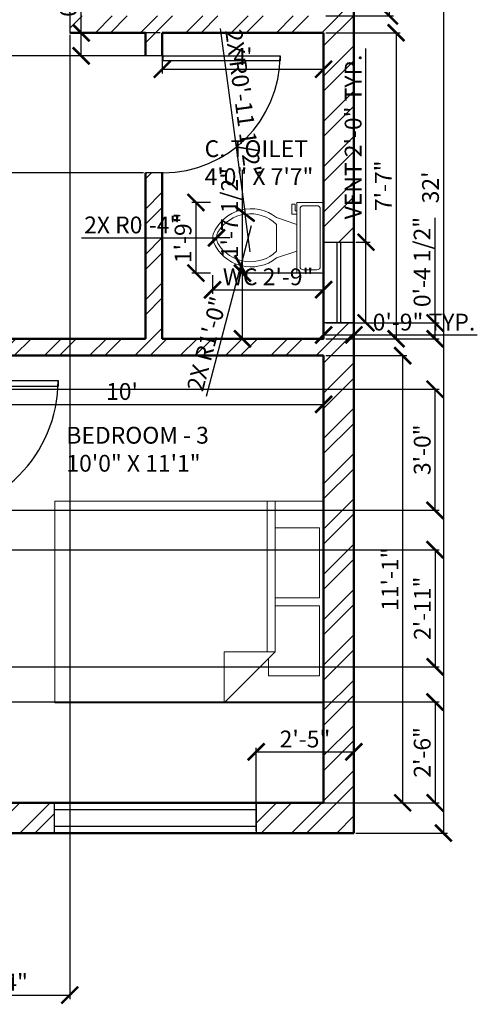
# Model space of a CAD drawing. Units: inches. Extents: x 683 to 1274, y 1901 to 2385.
# Tile 3 of 5: x 930 to 1066, y 1903 to 2196. Entities that reach past the tile are written whole.
import ezdxf

# ---------------------------------------------------------------- set-up
doc = ezdxf.new("R2010")
doc.units = ezdxf.units.IN
for name, color, linetype, lineweight in [('A-AREA-IDEN', 3, 'Continuous', 25), ('A-FLOR-FIXT', 2, 'Continuous', 18), ('A-FURN', 2, 'Continuous', 18), ('A-WALL-PATT', 8, 'Continuous', 13), ('DIM', 3, 'Continuous', 18), ('DOORS', 4, 'Continuous', 25), ('VENTILATOR', 11, 'Continuous', 25), ('walls', 6, 'Continuous', 50), ('WINDOWS', 30, 'Continuous', 25)]:
    doc.layers.add(name, color=color, linetype=linetype, lineweight=lineweight)
doc.styles.get("Standard").update_dxf_attribs({"font": 'arial.ttf'})
doc.dimstyles.new('ISO-25', dxfattribs={"dimtxt": 5, "dimasz": 5, "dimexe": 1.25, "dimexo": 0.625, "dimtad": 1, "dimdec": 1, "dimlunit": 4, "dimtxsty": 'Standard', "dimblk": 'ARCHTICK', "dimcen": 2.5, "dimadec": 0, "dimazin": 0, "dimtfac": 1, "dimtdec": 1, "dimtmove": 0, "dimatfit": 3, "dimfxl": 1, "dimarcsym": 0})

# ---------------------------------------------------------------- blocks, each defined once
blk = doc.blocks.new('Toilet - top')
for p, q in [((9.5, -6), (9.5, -2)), ((-10, -8.5), (-8, -8.5)), ((-10, -9.5), (-10, -8.5)), ((-8, -8.5), (-8, -8)), ((-7, -8), (-7, -9.5)), ((-4, -8), (-6, -14)), ((4, -8), (6, -14)), ((-7, -9.5), (-10, -9.5)), ((4, -14), (-4, -14))]:
    blk.add_line(p, q)
blk.add_lwpolyline([(10.5, -8), (10.5, 0), (-10.5, 0), (-10.5, -8)], close=True)
for points in [[(-9.5, -2), (-9.5, -6)], [(8.5, -1), (-8.5, -1)], [(-8.5, -7), (8.5, -7)]]:
    blk.add_lwpolyline(points)
for centre, radius, start, end in [((-8.62, -1.88), 0.884, 81.8699, 188.1301), ((8.62, -1.88), 0.884, 351.8699, 98.1301), ((-8.62, -6.12), 0.884, 171.8699, 278.1301), ((8.62, -6.12), 0.884, 261.8699, 8.1301), ((3.52, -21.58), 12.17, 141.4691, 247.9714), ((4.2, -21.82), 11.33, 136.3677, 238.9468), ((-3.52, -21.58), 12.17, 292.0284, 38.5307), ((-4.2, -21.82), 11.33, 301.053, 43.6321), ((0, -27.88), 4, 245.7318, 294.2682), ((0, -29), 4, 254.8605, 285.1395)]:
    blk.add_arc(centre, radius, start, end)
blk = doc.blocks.new('Bed - Queen')
for p, q in [((0, -80.00003), (0, 0)), ((0, 0), (59.99999, 0)), ((59.99999, 0), (59.99999, -80.00003)), ((7.99999, -1.2), (28.79998, -1.2)), ((7.99999, -14.4), (7.99999, -1.2)), ((28.79998, -1.2), (28.79998, -14.4)), ((31.19999, -1.2), (51.99999, -1.2)), ((31.19999, -14.4), (31.19999, -1.2)), ((51.99999, -1.2), (51.99999, -16.4)), ((0, -14.4), (44.8, -14.4)), ((59.99999, -29.6), (44.8, -14.4)), ((44.8, -14.4), (44.8, -29.6)), ((44.8, -16.8), (0, -16.8)), ((51.99999, -16.4), (46.79936, -16.4)), ((44.8, -29.6), (59.99999, -29.6)), ((59.99999, -80.00003), (0, -80.00003))]:
    blk.add_line(p, q)
blk = doc.blocks.new('_ArchTick')
at = {"color": 0, "linetype": 'ByBlock', "const_width": 0.15}
blk.add_lwpolyline([(-0.5, -0.5), (0.5, 0.5)], dxfattribs=at)
blk = doc.blocks.new('*D7')
at = {"layer": 'Defpoints', "color": 0, "transparency": 16777216}
for p in [(1029.42, 2337.78), (1029.42, 1953.78), (1056.05, 1953.78)]:
    blk.add_point(p, dxfattribs=at)
at = {"layer": 'DIM', "color": 0, "lineweight": -2, "transparency": 16777216}
for p, q in [((1030.04, 2337.78), (1057.3, 2337.78)), ((1056.05, 2337.78), (1056.05, 1953.78)), ((1030.04, 1953.78), (1057.3, 1953.78))]:
    blk.add_line(p, q, dxfattribs=at)
at = {"layer": 'DIM', "color": 0, "lineweight": -2, "transparency": 16777216, "xscale": 5, "yscale": 5, "zscale": 5}
for p, rotation in [((1056.05, 2337.78), 90), ((1056.05, 1953.78), 270)]:
    blk.add_blockref('_ArchTick', p, dxfattribs=dict(at, rotation=rotation))
at = {"layer": 'DIM', "color": 0, "transparency": 16777216, "insert": (1052.87, 2145.78), "char_height": 5, "attachment_point": 5, "rotation": 90}
blk.add_mtext("32'", dxfattribs=at)
blk = doc.blocks.new('*D8')
at = {"layer": 'Defpoints', "color": 0, "transparency": 16777216}
for p in [(900.42, 2095.78), (1020.42, 2095.78), (1020.42, 2081.28)]:
    blk.add_point(p, dxfattribs=at)
at = {"layer": 'DIM', "color": 0, "lineweight": -2, "transparency": 16777216}
for p, q in [((900.42, 2095.16), (900.42, 2080.03)), ((1020.42, 2095.16), (1020.42, 2080.03)), ((900.42, 2081.28), (1020.42, 2081.28))]:
    blk.add_line(p, q, dxfattribs=at)
at = {"layer": 'DIM', "color": 0, "lineweight": -2, "transparency": 16777216, "xscale": 5, "yscale": 5, "zscale": 5, "rotation": 180}
blk.add_blockref('_ArchTick', (900.42, 2081.28), dxfattribs=at)
at = {"layer": 'DIM', "color": 0, "lineweight": -2, "transparency": 16777216, "xscale": 5, "yscale": 5, "zscale": 5}
blk.add_blockref('_ArchTick', (1020.42, 2081.28), dxfattribs=at)
at = {"layer": 'DIM', "color": 0, "transparency": 16777216, "insert": (960.42, 2084.46), "char_height": 5, "attachment_point": 5}
blk.add_mtext("10'", dxfattribs=at)
blk = doc.blocks.new('*D11')
at = {"layer": 'Defpoints', "color": 0, "transparency": 16777216}
for p in [(972.42, 2191.78), (1020.42, 2191.78), (1020.42, 2180.94)]:
    blk.add_point(p, dxfattribs=at)
at = {"layer": 'DIM', "color": 0, "lineweight": -2, "transparency": 16777216}
for p, q in [((972.42, 2191.16), (972.42, 2179.69)), ((1020.42, 2191.16), (1020.42, 2179.69)), ((972.42, 2180.94), (1020.42, 2180.94))]:
    blk.add_line(p, q, dxfattribs=at)
at = {"layer": 'DIM', "color": 0, "lineweight": -2, "transparency": 16777216, "xscale": 5, "yscale": 5, "zscale": 5, "rotation": 180}
blk.add_blockref('_ArchTick', (972.42, 2180.94), dxfattribs=at)
at = {"layer": 'DIM', "color": 0, "lineweight": -2, "transparency": 16777216, "xscale": 5, "yscale": 5, "zscale": 5}
blk.add_blockref('_ArchTick', (1020.42, 2180.94), dxfattribs=at)
at = {"layer": 'DIM', "color": 0, "transparency": 16777216, "insert": (996.42, 2184.07), "char_height": 5, "attachment_point": 5}
blk.add_mtext("4'", dxfattribs=at)
blk = doc.blocks.new('VENTILATOR')
at = {"layer": 'VENTILATOR'}
for p, q in [((1084.96, 2166.43), (1093.96, 2166.43)), ((1084.96, 2142.43), (1084.96, 2166.43)), ((1088.96, 2142.43), (1088.96, 2166.43)), ((1089.96, 2166.43), (1089.96, 2142.43)), ((1093.96, 2166.43), (1093.96, 2142.43)), ((1093.96, 2142.43), (1084.96, 2142.43))]:
    blk.add_line(p, q, dxfattribs=at)
blk = doc.blocks.new('W1')
at = {"layer": 'WINDOWS'}
for p, q in [((1078.63, 2170.04), (1087.63, 2170.04)), ((1078.63, 2110.04), (1078.63, 2170.04)), ((1080.63, 2110.04), (1080.63, 2170.04)), ((1085.63, 2170.04), (1085.63, 2110.04)), ((1087.63, 2170.04), (1087.63, 2110.04)), ((1087.63, 2110.04), (1078.63, 2110.04))]:
    blk.add_line(p, q, dxfattribs=at)
blk = doc.blocks.new('*U18')
for p, q in [((0, 0), (0, -6)), ((40, 0), (40, -6))]:
    blk.add_line(p, q)
blk.add_lwpolyline([(0, 0), (0, 40), (1.75, 40), (1.75, 0)], close=True)
blk.add_arc((0, 0), 40, 0, 90)
blk = doc.blocks.new('*D20')
at = {"layer": 'Defpoints', "color": 0, "transparency": 16777216}
for p in [(1020.42, 2328.78), (1040, 2328.78), (1020.42, 2196.78)]:
    blk.add_point(p, dxfattribs=at)
at = {"layer": 'DIM', "color": 0, "lineweight": -2, "transparency": 16777216}
for p, q in [((1021.04, 2328.78), (1041.25, 2328.78)), ((1040, 2196.78), (1040, 2328.78)), ((1021.04, 2196.78), (1041.25, 2196.78))]:
    blk.add_line(p, q, dxfattribs=at)
at = {"layer": 'DIM', "color": 0, "lineweight": -2, "transparency": 16777216, "xscale": 5, "yscale": 5, "zscale": 5}
for p, rotation in [((1040, 2328.78), 90), ((1040, 2196.78), 270)]:
    blk.add_blockref('_ArchTick', p, dxfattribs=dict(at, rotation=rotation))
at = {"layer": 'DIM', "color": 0, "transparency": 16777216, "insert": (1036.87, 2262.78), "char_height": 5, "attachment_point": 5, "rotation": 90}
blk.add_mtext("11'", dxfattribs=at)
blk = doc.blocks.new('*D21')
at = {"layer": 'Defpoints', "color": 0, "transparency": 16777216}
for p in [(1020.42, 2191.78), (1020.42, 2100.78), (1041.97, 2100.78)]:
    blk.add_point(p, dxfattribs=at)
at = {"layer": 'DIM', "color": 0, "lineweight": -2, "transparency": 16777216}
for p, q in [((1021.04, 2191.78), (1043.22, 2191.78)), ((1041.97, 2191.78), (1041.97, 2100.78)), ((1021.04, 2100.78), (1043.22, 2100.78))]:
    blk.add_line(p, q, dxfattribs=at)
at = {"layer": 'DIM', "color": 0, "lineweight": -2, "transparency": 16777216, "xscale": 5, "yscale": 5, "zscale": 5}
for p, rotation in [((1041.97, 2191.78), 90), ((1041.97, 2100.78), 270)]:
    blk.add_blockref('_ArchTick', p, dxfattribs=dict(at, rotation=rotation))
at = {"layer": 'DIM', "color": 0, "transparency": 16777216, "insert": (1038.84, 2146.28), "char_height": 5, "attachment_point": 5, "rotation": 90}
blk.add_mtext('7\'-7"', dxfattribs=at)
blk = doc.blocks.new('*D22')
at = {"layer": 'Defpoints', "color": 0, "transparency": 16777216}
for p in [(1020.42, 2095.78), (1020.42, 1962.78), (1043.93, 1962.78)]:
    blk.add_point(p, dxfattribs=at)
at = {"layer": 'DIM', "color": 0, "lineweight": -2, "transparency": 16777216}
for p, q in [((1021.04, 2095.78), (1045.18, 2095.78)), ((1043.93, 2095.78), (1043.93, 1962.78)), ((1021.04, 1962.78), (1045.18, 1962.78))]:
    blk.add_line(p, q, dxfattribs=at)
at = {"layer": 'DIM', "color": 0, "lineweight": -2, "transparency": 16777216, "xscale": 5, "yscale": 5, "zscale": 5}
for p, rotation in [((1043.93, 2095.78), 90), ((1043.93, 1962.78), 270)]:
    blk.add_blockref('_ArchTick', p, dxfattribs=dict(at, rotation=rotation))
at = {"layer": 'DIM', "color": 0, "transparency": 16777216, "insert": (1040.79, 2029.28), "char_height": 5, "attachment_point": 5, "rotation": 90}
blk.add_mtext('11\'-1"', dxfattribs=at)
blk = doc.blocks.new('*D31')
at = {"layer": 'Defpoints', "color": 0, "transparency": 16777216}
for p in [(1029.42, 2129.51), (1033.02, 2129.51), (1029.42, 2105.51)]:
    blk.add_point(p, dxfattribs=at)
at = {"layer": 'DIM', "color": 0, "lineweight": -2, "transparency": 16777216}
for p, q in [((1033.02, 2129.51), (1033.02, 2187.07)), ((1030.04, 2129.51), (1034.27, 2129.51)), ((1033.02, 2105.51), (1033.02, 2129.51)), ((1030.04, 2105.51), (1034.27, 2105.51))]:
    blk.add_line(p, q, dxfattribs=at)
at = {"layer": 'DIM', "color": 0, "lineweight": -2, "transparency": 16777216, "xscale": 5, "yscale": 5, "zscale": 5}
for p, rotation in [((1033.02, 2129.51), 90), ((1033.02, 2105.51), 270)]:
    blk.add_blockref('_ArchTick', p, dxfattribs=dict(at, rotation=rotation))
at = {"layer": 'DIM', "color": 0, "transparency": 16777216, "insert": (1029.84, 2160.79), "char_height": 5, "attachment_point": 5, "rotation": 90}
blk.add_mtext('VENT 2\'-0" TYP.', dxfattribs=at)
blk = doc.blocks.new('*D32')
at = {"layer": 'Defpoints', "color": 0, "transparency": 16777216}
for p in [(1020.42, 2105.51), (1029.42, 2105.51), (1029.42, 2101.91)]:
    blk.add_point(p, dxfattribs=at)
at = {"layer": 'DIM', "color": 0, "lineweight": -2, "transparency": 16777216}
for p, q in [((1020.42, 2104.89), (1020.42, 2100.66)), ((1029.42, 2104.89), (1029.42, 2100.66)), ((1020.42, 2101.91), (1029.42, 2101.91)), ((1029.42, 2101.91), (1066.15, 2101.91))]:
    blk.add_line(p, q, dxfattribs=at)
at = {"layer": 'DIM', "color": 0, "lineweight": -2, "transparency": 16777216, "xscale": 5, "yscale": 5, "zscale": 5, "rotation": 180}
blk.add_blockref('_ArchTick', (1020.42, 2101.91), dxfattribs=at)
at = {"layer": 'DIM', "color": 0, "lineweight": -2, "transparency": 16777216, "xscale": 5, "yscale": 5, "zscale": 5}
blk.add_blockref('_ArchTick', (1029.42, 2101.91), dxfattribs=at)
at = {"layer": 'DIM', "color": 0, "transparency": 16777216, "insert": (1050.28, 2105.09), "char_height": 5, "attachment_point": 5}
blk.add_mtext('0\'-9" TYP.', dxfattribs=at)
blk = doc.blocks.new('*D37')
at = {"layer": 'Defpoints', "color": 0, "transparency": 16777216}
for p in [(987.37, 2120.31), (1020.42, 2120.31), (1020.42, 2115.35)]:
    blk.add_point(p, dxfattribs=at)
at = {"layer": 'DIM', "color": 0, "lineweight": -2, "transparency": 16777216}
for p, q in [((987.37, 2119.68), (987.37, 2114.1)), ((1020.42, 2119.68), (1020.42, 2114.1)), ((987.37, 2115.35), (1020.42, 2115.35))]:
    blk.add_line(p, q, dxfattribs=at)
at = {"layer": 'DIM', "color": 0, "lineweight": -2, "transparency": 16777216, "xscale": 5, "yscale": 5, "zscale": 5, "rotation": 180}
blk.add_blockref('_ArchTick', (987.37, 2115.35), dxfattribs=at)
at = {"layer": 'DIM', "color": 0, "lineweight": -2, "transparency": 16777216, "xscale": 5, "yscale": 5, "zscale": 5}
blk.add_blockref('_ArchTick', (1020.42, 2115.35), dxfattribs=at)
at = {"layer": 'DIM', "color": 0, "transparency": 16777216, "insert": (1003.9, 2118.56), "char_height": 5, "attachment_point": 5}
blk.add_mtext('WC 2\'-9"', dxfattribs=at)
blk = doc.blocks.new('*D38')
at = {"layer": 'Defpoints', "color": 0, "transparency": 16777216}
for p in [(987.37, 2141.31), (982.42, 2120.31), (987.37, 2120.31)]:
    blk.add_point(p, dxfattribs=at)
at = {"layer": 'DIM', "color": 0, "lineweight": -2, "transparency": 16777216}
for p, q in [((986.75, 2141.31), (981.17, 2141.31)), ((982.42, 2141.31), (982.42, 2120.31)), ((986.75, 2120.31), (981.17, 2120.31))]:
    blk.add_line(p, q, dxfattribs=at)
at = {"layer": 'DIM', "color": 0, "lineweight": -2, "transparency": 16777216, "xscale": 5, "yscale": 5, "zscale": 5}
for p, rotation in [((982.42, 2141.31), 90), ((982.42, 2120.31), 270)]:
    blk.add_blockref('_ArchTick', p, dxfattribs=dict(at, rotation=rotation))
at = {"layer": 'DIM', "color": 0, "transparency": 16777216, "insert": (979.24, 2130.81), "char_height": 5, "attachment_point": 5, "rotation": 90}
blk.add_mtext('1\'-9"', dxfattribs=at)
blk = doc.blocks.new('*D42')
at = {"layer": 'Defpoints', "color": 0, "transparency": 16777216}
for p in [(826.42, 2038.04), (826.42, 2003.23), (1053.57, 2003.23)]:
    blk.add_point(p, dxfattribs=at)
at = {"layer": 'DIM', "color": 0, "lineweight": -2, "transparency": 16777216}
for p, q in [((827.04, 2038.04), (1054.82, 2038.04)), ((1053.57, 2038.04), (1053.57, 2003.23)), ((827.04, 2003.23), (1054.82, 2003.23))]:
    blk.add_line(p, q, dxfattribs=at)
at = {"layer": 'DIM', "color": 0, "lineweight": -2, "transparency": 16777216, "xscale": 5, "yscale": 5, "zscale": 5}
for p, rotation in [((1053.57, 2038.04), 90), ((1053.57, 2003.23), 270)]:
    blk.add_blockref('_ArchTick', p, dxfattribs=dict(at, rotation=rotation))
at = {"layer": 'DIM', "color": 0, "transparency": 16777216, "insert": (1050.43, 2020.64), "char_height": 5, "attachment_point": 5, "rotation": 90}
blk.add_mtext('2\'-11"', dxfattribs=at)
blk = doc.blocks.new('*D43')
at = {"layer": 'Defpoints', "color": 0, "transparency": 16777216}
for p in [(693.27, 2184.95), (967.42, 2184.95), (967.42, 2150.14)]:
    blk.add_point(p, dxfattribs=at)
at = {"layer": 'DIM', "color": 0, "lineweight": -2, "transparency": 16777216}
for p, q in [((966.79, 2184.95), (692.02, 2184.95)), ((693.27, 2150.14), (693.27, 2184.95)), ((966.79, 2150.14), (692.02, 2150.14))]:
    blk.add_line(p, q, dxfattribs=at)
at = {"layer": 'DIM', "color": 0, "lineweight": -2, "transparency": 16777216, "xscale": 5, "yscale": 5, "zscale": 5}
for p, rotation in [((693.27, 2184.95), 90), ((693.27, 2150.14), 270)]:
    blk.add_blockref('_ArchTick', p, dxfattribs=dict(at, rotation=rotation))
at = {"layer": 'DIM', "color": 0, "transparency": 16777216, "insert": (690.13, 2167.54), "char_height": 5, "attachment_point": 5, "rotation": 90}
blk.add_mtext('2\'-11"', dxfattribs=at)
blk = doc.blocks.new('*D46')
at = {"layer": 'Defpoints', "color": 0, "transparency": 16777216}
for p in [(904.89, 2191.78), (944.89, 2191.78), (944.89, 1905.63)]:
    blk.add_point(p, dxfattribs=at)
at = {"layer": 'DIM', "color": 0, "lineweight": -2, "transparency": 16777216}
for p, q in [((904.89, 2191.16), (904.89, 1904.38)), ((944.89, 2191.16), (944.89, 1904.38)), ((904.89, 1905.63), (944.89, 1905.63))]:
    blk.add_line(p, q, dxfattribs=at)
at = {"layer": 'DIM', "color": 0, "lineweight": -2, "transparency": 16777216, "xscale": 5, "yscale": 5, "zscale": 5, "rotation": 180}
blk.add_blockref('_ArchTick', (904.89, 1905.63), dxfattribs=at)
at = {"layer": 'DIM', "color": 0, "lineweight": -2, "transparency": 16777216, "xscale": 5, "yscale": 5, "zscale": 5}
blk.add_blockref('_ArchTick', (944.89, 1905.63), dxfattribs=at)
at = {"layer": 'DIM', "color": 0, "transparency": 16777216, "insert": (924.89, 1908.81), "char_height": 5, "attachment_point": 5}
blk.add_mtext('3\'-4"', dxfattribs=at)
blk = doc.blocks.new('*D49')
at = {"layer": 'Defpoints', "color": 0, "transparency": 16777216}
for p in [(802.42, 2085.78), (1053.57, 2085.78), (802.42, 2049.78)]:
    blk.add_point(p, dxfattribs=at)
at = {"layer": 'DIM', "color": 0, "lineweight": -2, "transparency": 16777216}
for p, q in [((803.04, 2085.78), (1054.82, 2085.78)), ((1053.57, 2049.78), (1053.57, 2085.78)), ((803.04, 2049.78), (1054.82, 2049.78))]:
    blk.add_line(p, q, dxfattribs=at)
at = {"layer": 'DIM', "color": 0, "lineweight": -2, "transparency": 16777216, "xscale": 5, "yscale": 5, "zscale": 5}
for p, rotation in [((1053.57, 2085.78), 90), ((1053.57, 2049.78), 270)]:
    blk.add_blockref('_ArchTick', p, dxfattribs=dict(at, rotation=rotation))
at = {"layer": 'DIM', "color": 0, "transparency": 16777216, "insert": (1050.39, 2067.78), "char_height": 5, "attachment_point": 5, "rotation": 90}
blk.add_mtext('3\'-0"', dxfattribs=at)
blk = doc.blocks.new('*D53')
at = {"layer": 'Defpoints', "color": 0, "transparency": 16777216}
for p in [(1029.42, 1977.93), (1000.32, 1953.78), (1029.42, 1953.78)]:
    blk.add_point(p, dxfattribs=at)
at = {"layer": 'DIM', "color": 0, "lineweight": -2, "transparency": 16777216}
for p, q in [((1000.32, 1954.41), (1000.32, 1979.18)), ((1000.32, 1977.93), (1029.42, 1977.93)), ((1029.42, 1954.41), (1029.42, 1979.18))]:
    blk.add_line(p, q, dxfattribs=at)
at = {"layer": 'DIM', "color": 0, "lineweight": -2, "transparency": 16777216, "xscale": 5, "yscale": 5, "zscale": 5, "rotation": 180}
blk.add_blockref('_ArchTick', (1000.32, 1977.93), dxfattribs=at)
at = {"layer": 'DIM', "color": 0, "lineweight": -2, "transparency": 16777216, "xscale": 5, "yscale": 5, "zscale": 5}
blk.add_blockref('_ArchTick', (1029.42, 1977.93), dxfattribs=at)
at = {"layer": 'DIM', "color": 0, "transparency": 16777216, "insert": (1014.87, 1981.11), "char_height": 5, "attachment_point": 5}
blk.add_mtext('2\'-5"', dxfattribs=at)
blk = doc.blocks.new('*D54')
at = {"layer": 'Defpoints', "color": 0, "transparency": 16777216}
for p in [(1020.42, 2105.51), (1053.57, 2105.51), (1020.42, 2100.78)]:
    blk.add_point(p, dxfattribs=at)
at = {"layer": 'DIM', "color": 0, "lineweight": -2, "transparency": 16777216}
for p, q in [((1053.57, 2105.51), (1053.57, 2136.7)), ((1021.04, 2105.51), (1054.82, 2105.51)), ((1053.57, 2100.78), (1053.57, 2105.51)), ((1021.04, 2100.78), (1054.82, 2100.78))]:
    blk.add_line(p, q, dxfattribs=at)
at = {"layer": 'DIM', "color": 0, "lineweight": -2, "transparency": 16777216, "xscale": 5, "yscale": 5, "zscale": 5}
for p, rotation in [((1053.57, 2105.51), 90), ((1053.57, 2100.78), 270)]:
    blk.add_blockref('_ArchTick', p, dxfattribs=dict(at, rotation=rotation))
at = {"layer": 'DIM', "color": 0, "transparency": 16777216, "insert": (1050.36, 2123.61), "char_height": 5, "attachment_point": 5, "rotation": 90}
blk.add_mtext('0\'-4 1/2"', dxfattribs=at)
blk = doc.blocks.new('*D59')
at = {"layer": 'Defpoints', "color": 0, "transparency": 16777216}
for p in [(821.42, 1992.78), (821.42, 1962.78), (1053.57, 1962.78)]:
    blk.add_point(p, dxfattribs=at)
at = {"layer": 'DIM', "color": 0, "lineweight": -2, "transparency": 16777216}
for p, q in [((822.04, 1992.78), (1054.82, 1992.78)), ((1053.57, 1992.78), (1053.57, 1962.78)), ((822.04, 1962.78), (1054.82, 1962.78))]:
    blk.add_line(p, q, dxfattribs=at)
at = {"layer": 'DIM', "color": 0, "lineweight": -2, "transparency": 16777216, "xscale": 5, "yscale": 5, "zscale": 5}
for p, rotation in [((1053.57, 1992.78), 90), ((1053.57, 1962.78), 270)]:
    blk.add_blockref('_ArchTick', p, dxfattribs=dict(at, rotation=rotation))
at = {"layer": 'DIM', "color": 0, "transparency": 16777216, "insert": (1050.39, 1977.78), "char_height": 5, "attachment_point": 5, "rotation": 90}
blk.add_mtext('2\'-6"', dxfattribs=at)
blk = doc.blocks.new('*D60')
at = {"layer": 'Defpoints', "color": 0, "transparency": 16777216}
for p in [(996.27, 2120.31), (1020.42, 2120.31), (1020.42, 2100.78)]:
    blk.add_point(p, dxfattribs=at)
at = {"layer": 'DIM', "color": 0, "lineweight": -2, "transparency": 16777216}
for p, q in [((996.27, 2120.31), (996.27, 2151.03)), ((1019.79, 2120.31), (995.02, 2120.31)), ((996.27, 2100.78), (996.27, 2120.31)), ((1019.79, 2100.78), (995.02, 2100.78))]:
    blk.add_line(p, q, dxfattribs=at)
at = {"layer": 'DIM', "color": 0, "lineweight": -2, "transparency": 16777216, "xscale": 5, "yscale": 5, "zscale": 5}
for p, rotation in [((996.27, 2120.31), 90), ((996.27, 2100.78), 270)]:
    blk.add_blockref('_ArchTick', p, dxfattribs=dict(at, rotation=rotation))
at = {"layer": 'DIM', "color": 0, "transparency": 16777216, "insert": (993.06, 2138.17), "char_height": 5, "attachment_point": 5, "rotation": 90}
blk.add_mtext('1\'-7 1/2"', dxfattribs=at)
blk = doc.blocks.new('*D67')
at = {"layer": 'Defpoints', "color": 0, "transparency": 16777216}
for p in [(948.27, 2191.78), (972.42, 2191.78), (972.42, 2184.95)]:
    blk.add_point(p, dxfattribs=at)
at = {"layer": 'DIM', "color": 0, "lineweight": -2, "transparency": 16777216}
for p, q in [((948.27, 2191.78), (948.27, 2211.32)), ((971.79, 2191.78), (947.02, 2191.78)), ((948.27, 2184.95), (948.27, 2191.78)), ((971.79, 2184.95), (947.02, 2184.95))]:
    blk.add_line(p, q, dxfattribs=at)
at = {"layer": 'DIM', "color": 0, "lineweight": -2, "transparency": 16777216, "xscale": 5, "yscale": 5, "zscale": 5}
for p, rotation in [((948.27, 2191.78), 90), ((948.27, 2184.95), 270)]:
    blk.add_blockref('_ArchTick', p, dxfattribs=dict(at, rotation=rotation))
at = {"layer": 'DIM', "color": 0, "transparency": 16777216, "insert": (945.09, 2204.05), "char_height": 5, "attachment_point": 5, "rotation": 90}
blk.add_mtext('0\'-7"', dxfattribs=at)
blk = doc.blocks.new('*D68')
at = {"layer": 'Defpoints', "color": 0, "transparency": 16777216}
for p in [(988.54, 2130.81), (992.54, 2130.81)]:
    blk.add_point(p, dxfattribs=at)
at = {"layer": 'DIM', "color": 0, "lineweight": -2, "transparency": 16777216}
for p in [(948.39, 2130.8), (992.54, 2130.81)]:
    blk.add_line(p, (988.54, 2130.81), dxfattribs=at)
at = {"layer": 'DIM', "color": 0, "lineweight": -2, "transparency": 16777216, "xscale": 5, "yscale": 5, "zscale": 5, "rotation": 0.0010170000918173}
blk.add_blockref('_ArchTick', (988.54, 2130.81), dxfattribs=at)
at = {"layer": 'DIM', "color": 0, "transparency": 16777216, "insert": (963.47, 2133.98), "char_height": 5, "attachment_point": 5, "rotation": 0.001}
blk.add_mtext('2X R0\'-4"', dxfattribs=at)
blk = doc.blocks.new('*D69')
at = {"layer": 'Defpoints', "color": 0, "transparency": 16777216}
for p in [(998.84, 2134.32), (995.75, 2122.55)]:
    blk.add_point(p, dxfattribs=at)
at = {"layer": 'DIM', "color": 0, "lineweight": -2, "transparency": 16777216}
for p in [(998.84, 2134.32), (985.54, 2083.72)]:
    blk.add_line(p, (995.75, 2122.55), dxfattribs=at)
at = {"layer": 'DIM', "color": 0, "lineweight": -2, "transparency": 16777216, "xscale": 5, "yscale": 5, "zscale": 5, "rotation": 75.27949628550273}
blk.add_blockref('_ArchTick', (995.75, 2122.55), dxfattribs=at)
at = {"layer": 'DIM', "color": 0, "transparency": 16777216, "insert": (986.3, 2099.11), "char_height": 5, "attachment_point": 5, "rotation": 75.2795}
blk.add_mtext('2X R1\'-0"', dxfattribs=at)
blk = doc.blocks.new('*D70')
at = {"layer": 'Defpoints', "color": 0, "transparency": 16777216}
for p in [(997.09, 2137.83), (998.6, 2126.61)]:
    blk.add_point(p, dxfattribs=at)
at = {"layer": 'DIM', "color": 0, "lineweight": -2, "transparency": 16777216}
for p in [(989.67, 2193.03), (998.6, 2126.61)]:
    blk.add_line(p, (997.09, 2137.83), dxfattribs=at)
at = {"layer": 'DIM', "color": 0, "lineweight": -2, "transparency": 16777216, "xscale": 5, "yscale": 5, "zscale": 5, "rotation": 277.6558557887796}
blk.add_blockref('_ArchTick', (997.09, 2137.83), dxfattribs=at)
at = {"layer": 'DIM', "color": 0, "transparency": 16777216, "insert": (995.9, 2170.81), "char_height": 5, "attachment_point": 5, "rotation": 277.6559}
blk.add_mtext('2X R0\'-11 1/2"', dxfattribs=at)

msp = doc.modelspace()

# ---------------------------------------------------------------- hatches: boundary and pattern name
at = {"layer": 'A-WALL-PATT'}
h = msp.add_hatch(dxfattribs=at)
h.set_pattern_fill('ANSI32', color=256)
h.paths.add_polyline_path([(717.42, 2337.78), (717.42, 2300.95), (726.42, 2300.95), (726.42, 2328.78), (895.42, 2328.78), (895.42, 2196.78), (890.48, 2196.78), (890.48, 2191.78), (904.89, 2191.78), (904.89, 2196.78), (900.42, 2196.78), (900.42, 2328.78), (1020.42, 2328.78), (1020.42, 2303.09), (1029.42, 2303.09), (1029.42, 2337.78)])
h.paths.add_polyline_path([(1020.42, 2196.78), (944.89, 2196.78), (944.89, 2191.78), (967.42, 2191.78), (967.42, 2184.95), (972.42, 2184.95), (972.42, 2191.78), (1020.42, 2191.78), (1020.42, 2129.51), (1029.42, 2129.51), (1029.42, 2243.09), (1020.42, 2243.09)])
h.paths.add_polyline_path([(1029.42, 2105.51), (1020.42, 2105.51), (1020.42, 2100.78), (972.42, 2100.78), (972.42, 2150.14), (967.42, 2150.14), (967.42, 2100.78), (895.42, 2100.78), (895.42, 2088.36), (900.42, 2088.36), (900.42, 2095.78), (1020.42, 2095.78), (1020.42, 1962.78), (1000.32, 1962.78), (1000.32, 1953.78), (1029.42, 1953.78)])
h.paths.add_polyline_path([(940.32, 1953.78), (940.32, 1962.78), (900.42, 1962.78), (900.42, 2048.36), (895.42, 2048.36), (895.42, 1962.78), (882.7, 1962.78), (882.7, 1959.78), (882.7, 1953.78)])
h.paths.add_polyline_path([(790.86, 1953.78), (790.86, 1962.78), (726.42, 1962.78), (726.42, 1980.18), (717.42, 1980.18), (717.42, 1953.78)])
h.paths.add_polyline_path([(842.7, 1953.78), (842.7, 1959.78, -0.01877), (842.81, 1962.78), (826.42, 1962.78), (826.42, 2003.23), (821.42, 2003.23), (821.42, 1962.78), (814.86, 1962.78), (814.86, 1953.78)])
h.paths.add_polyline_path([(726.42, 2196.78), (726.42, 2240.95), (717.42, 2240.95), (717.42, 2167.98), (726.42, 2167.98), (726.42, 2191.78), (850.48, 2191.78), (850.48, 2196.78)])

# ---------------------------------------------------------------- linework, layer by layer
at = {"layer": 'walls'}
for p, q in [((1029.42, 2337.78), (1029.42, 1953.78)), ((944.89, 2191.78), (967.42, 2191.78)), ((967.42, 2191.78), (967.42, 2184.95)), ((972.42, 2191.78), (972.42, 2184.95)), ((972.42, 2191.78), (1020.42, 2191.78)), ((1020.42, 2191.78), (1020.42, 2100.78)), ((967.42, 2150.14), (967.42, 2100.78)), ((972.42, 2150.14), (972.42, 2100.78)), ((895.42, 2100.78), (967.42, 2100.78)), ((972.42, 2100.78), (1020.42, 2100.78)), ((900.42, 2095.78), (1020.42, 2095.78)), ((1020.42, 2095.78), (1020.42, 1962.78)), ((1020.42, 1962.78), (900.42, 1962.78)), ((1029.42, 1953.78), (717.42, 1953.78))]:
    msp.add_line(p, q, dxfattribs=at)

# ---------------------------------------------------------------- block references
at = {"layer": 'A-FLOR-FIXT', "rotation": 270}
msp.add_blockref('Toilet - top', (1020.42, 2130.81), dxfattribs=at)
at = {"layer": 'A-FURN', "rotation": 270}
msp.add_blockref('Bed - Queen', (1020.42, 2052.52), dxfattribs=at)
at = {"layer": 'DOORS'}
msp.add_blockref('*U18', (904.89, 2197.78), dxfattribs=at)
at = {"layer": 'DOORS', "xscale": 0.8703088381272287, "yscale": 0.8703088381272287, "zscale": 0.8703088381272287, "rotation": 270}
msp.add_blockref('*U18', (972.64, 2184.95), dxfattribs=at)
at = {"layer": 'DOORS', "rotation": 270}
msp.add_blockref('*U18', (901.42, 2088.36), dxfattribs=at)
at = {"layer": 'VENTILATOR'}
msp.add_blockref('VENTILATOR', (-64.54, -36.91), dxfattribs=at)
at = {"layer": 'WINDOWS', "rotation": 270}
msp.add_blockref('W1', (-1169.72, 3041.41), dxfattribs=at)

# ---------------------------------------------------------------- texts
at = {"layer": 'A-AREA-IDEN', "char_height": 5, "attachment_point": 1}
for s, width, insert in [('{C. TOILET  \\P4\'0" X 7\'7"}', 34.6524, (985, 2159.81)), ('{BEDROOM - 3 \\P10\'0" X 11\'1"}', 48.7562, (943.87, 2074.59))]:
    msp.add_mtext_dynamic_manual_height_columns(s, width=width, gutter_width=12.5, heights=[0], dxfattribs=dict(at, insert=insert))

# ---------------------------------------------------------------- dimensions: what is measured, and where the dimension line sits
at = {"layer": 'DIM'}
for base, p1, p2, angle, override, picture, middle in [((1056.05, 1953.78), (1029.42, 2337.78), (1029.42, 1953.78), 90, {"dimclrd": 0, "dimclre": 0, "dimclrt": 0}, '*D7', (1052.87, 2145.78)), ((1040, 2328.78), (1020.42, 2196.78), (1020.42, 2328.78), 90, {"dimclrd": 0, "dimclre": 0, "dimclrt": 0}, '*D20', (1036.87, 2262.78)), ((948.27, 2191.78), (972.42, 2184.95), (972.42, 2191.78), 90, {"dimdec": 1, "dimlfac": 1, "dimrnd": 0, "dimzin": 1, "dimdsep": 46, "dimlunit": 4, "dimfrac": 2}, '*D67', (945.09, 2204.05)), ((1041.97, 2100.78), (1020.42, 2191.78), (1020.42, 2100.78), 90, {"dimclrd": 0, "dimclre": 0, "dimclrt": 0}, '*D21', (1038.84, 2146.28)), ((693.27, 2184.95), (967.42, 2150.14), (967.42, 2184.95), 90, {"dimdec": 1, "dimlfac": 1, "dimrnd": 0, "dimzin": 1, "dimdsep": 46, "dimlunit": 4, "dimfrac": 2}, '*D43', (690.13, 2167.54)), ((996.27, 2120.31), (1020.42, 2100.78), (1020.42, 2120.31), 90, {"dimdec": 1, "dimlfac": 1, "dimrnd": 0, "dimzin": 1, "dimdsep": 46, "dimlunit": 4, "dimfrac": 2}, '*D60', (993.06, 2138.17)), ((982.42, 2120.31), (987.37, 2141.31), (987.37, 2120.31), 270, {"dimdec": 1, "dimlfac": 1, "dimrnd": 0, "dimzin": 1, "dimdsep": 46, "dimlunit": 4, "dimfrac": 2}, '*D38', (979.24, 2130.81)), ((1053.57, 2105.51), (1020.42, 2100.78), (1020.42, 2105.51), 90, {"dimdec": 1, "dimlfac": 1, "dimrnd": 0, "dimzin": 1, "dimdsep": 46, "dimlunit": 4, "dimfrac": 2}, '*D54', (1050.36, 2123.61)), ((1043.93, 1962.78), (1020.42, 2095.78), (1020.42, 1962.78), 90, {"dimclrd": 0, "dimclre": 0, "dimclrt": 0}, '*D22', (1040.79, 2029.28)), ((1053.57, 2085.78), (802.42, 2049.78), (802.42, 2085.78), 90, {"dimdec": 1, "dimlfac": 1, "dimrnd": 0, "dimzin": 1, "dimdsep": 46, "dimlunit": 4, "dimfrac": 2}, '*D49', (1050.39, 2067.78)), ((1053.57, 2003.23), (826.42, 2038.04), (826.42, 2003.23), 90, {"dimdec": 1, "dimlfac": 1, "dimrnd": 0, "dimzin": 1, "dimdsep": 46, "dimlunit": 4, "dimfrac": 2}, '*D42', (1050.43, 2020.64)), ((1053.57, 1962.78), (821.42, 1992.78), (821.42, 1962.78), 90, {"dimdec": 1, "dimlfac": 1, "dimrnd": 0, "dimzin": 1, "dimdsep": 46, "dimlunit": 4, "dimfrac": 2}, '*D59', (1050.39, 1977.78))]:
    dim = msp.add_linear_dim(base=base, p1=p1, p2=p2, angle=angle, dimstyle='ISO-25', override=override, dxfattribs=at)
    dim.commit()
    dim.dimension.update_dxf_attribs({"geometry": picture, "text_midpoint": middle})
for base, p1, p2, override, picture, middle in [((944.89, 1905.63), (904.89, 2191.78), (944.89, 2191.78), {"dimdec": 1, "dimlfac": 1, "dimrnd": 0, "dimzin": 1, "dimdsep": 46, "dimlunit": 4, "dimfrac": 2}, '*D46', (924.89, 1908.81)), ((1020.42, 2180.94), (972.42, 2191.78), (1020.42, 2191.78), {"dimclrd": 0, "dimclre": 0, "dimclrt": 0}, '*D11', (996.42, 2184.07)), ((1020.42, 2081.28), (900.42, 2095.78), (1020.42, 2095.78), {"dimclrd": 0, "dimclre": 0, "dimclrt": 0}, '*D8', (960.42, 2084.46)), ((1029.42, 1977.93), (1000.32, 1953.78), (1029.42, 1953.78), {"dimdec": 1, "dimlfac": 1, "dimrnd": 0, "dimzin": 1, "dimdsep": 46, "dimlunit": 4, "dimfrac": 2}, '*D53', (1014.87, 1981.11))]:
    dim = msp.add_linear_dim(base=base, p1=p1, p2=p2, dimstyle='ISO-25', override=override, dxfattribs=at)
    dim.commit()
    dim.dimension.update_dxf_attribs({"geometry": picture, "text_midpoint": middle})
for center, mpoint, picture, middle in [((998.6, 2126.61), (997.09, 2137.83), '*D70', (995.9, 2170.81)), ((992.54, 2130.81), (988.54, 2130.81), '*D68', (963.47, 2133.98)), ((998.84, 2134.32), (995.75, 2122.55), '*D69', (986.3, 2099.11))]:
    dim = msp.add_radius_dim(center=center, mpoint=mpoint, text='2X <>', dimstyle='ISO-25', override={"dimdec": 1, "dimlfac": 1, "dimrnd": 0, "dimzin": 1, "dimdsep": 46, "dimlunit": 4, "dimfrac": 2}, dxfattribs=at)
    dim.commit()
    dim.dimension.update_dxf_attribs({"geometry": picture, "text_midpoint": middle})
dim = msp.add_linear_dim(base=(1033.02, 2129.51), p1=(1029.42, 2105.51), p2=(1029.42, 2129.51), angle=90, text='VENT <> TYP.', dimstyle='ISO-25', override={"dimdec": 1, "dimlfac": 1, "dimrnd": 0, "dimzin": 1, "dimdsep": 46, "dimlunit": 4, "dimfrac": 2}, dxfattribs=at)
dim.commit()
dim.dimension.update_dxf_attribs({"geometry": '*D31', "text_midpoint": (1029.84, 2160.79)})
for base, p1, p2, text, picture, middle in [((1020.4197, 2115.3482), (987.3734, 2120.3051), (1020.4197, 2120.3051), 'WC <>', '*D37', (1003.8965, 2118.5584)), ((1029.42, 2101.91), (1020.42, 2105.51), (1029.42, 2105.51), '<> TYP.', '*D32', (1050.28, 2105.09))]:
    dim = msp.add_linear_dim(base=base, p1=p1, p2=p2, text=text, dimstyle='ISO-25', override={"dimdec": 1, "dimlfac": 1, "dimrnd": 0, "dimzin": 1, "dimdsep": 46, "dimlunit": 4, "dimfrac": 2}, dxfattribs=at)
    dim.commit()
    dim.dimension.update_dxf_attribs({"geometry": picture, "text_midpoint": middle})

doc.saveas('drawing.dxf')
